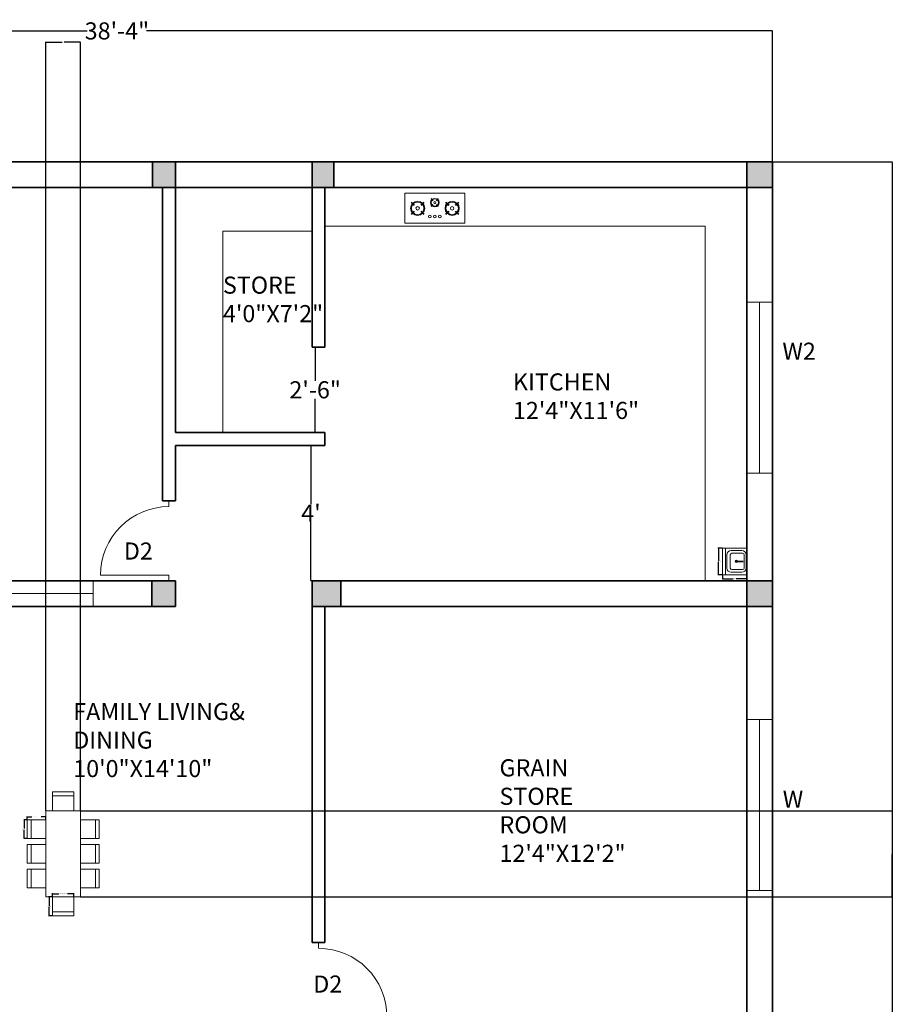
# Model space of a CAD drawing. Units: inches. Extents: x -36302355 to 648, y -221479757 to 75.
# Tile 37 of 37: x 341 to 648, y -271 to 75. Entities that reach past the tile are written whole.
import ezdxf

# ---------------------------------------------------------------- set-up
doc = ezdxf.new("R2010")
doc.units = ezdxf.units.IN
doc.header["$MEASUREMENT"] = 0
for name, color, linetype, lineweight in [('A-ANNO-DIMS', 2, 'Continuous', 18), ('A-ANNO-IDEN', 7, 'Continuous', 18), ('A-AREA-IDEN', 7, 'Continuous', 18), ('A-COLS', 7, 'Continuous', 35), ('A-COLS-PATT', 242, 'Continuous', 13), ('A-DOOR', 4, 'Continuous', 18), ('A-EQPM', 9, 'Continuous', 13), ('A-FLOR-CASE', 9, 'Continuous', 18), ('A-FLOR-FIXT', 9, 'Continuous', 18), ('A-FURN', 8, 'Continuous', 13), ('A-GLAZ', 142, 'Continuous', 18), ('A-WALL', 7, 'Continuous', 35)]:
    doc.layers.add(name, color=color, linetype=linetype, lineweight=lineweight)
doc.styles.get("Standard").update_dxf_attribs({"font": 'arial.ttf'})
doc.dimstyles.get("Standard").update_dxf_attribs({"dimtxt": 0.18, "dimasz": 0.18, "dimexe": 0.18, "dimexo": 0.0625, "dimgap": 0.09, "dimtad": 0, "dimtih": 1, "dimtoh": 1, "dimdec": 0, "dimzin": 0, "dimdsep": 46, "dimlunit": 3, "dimtxsty": 'Standard', "dimcen": 0.09, "dimadec": 0, "dimazin": 0, "dimtfac": 1, "dimtdec": 0, "dimtofl": 0, "dimtmove": 0, "dimatfit": 3, "dimfxl": 1, "dimtolj": 1, "dimtzin": 0, "dimarcsym": 0})

# ---------------------------------------------------------------- blocks, each defined once
blk = doc.blocks.new('*D2')
at = {"layer": 'A-ANNO-DIMS', "color": 0, "lineweight": -2, "transparency": 16777216}
for p, q in [((448.13, -74.52), (443.1, -74.52)), ((443.28, -74.7), (443.28, -95.18)), ((443.28, -121.84), (443.28, -101.36)), ((443.63, -122.02), (443.1, -122.02))]:
    blk.add_line(p, q, dxfattribs=at)
at = {"layer": 'A-ANNO-DIMS', "color": 0, "transparency": 16777216}
for points in [[(443.25, -74.7), (443.31, -74.7), (443.28, -74.52)], [(443.25, -121.84), (443.31, -121.84), (443.28, -122.02)]]:
    blk.add_solid(points, dxfattribs=at)
at = {"layer": 'Defpoints', "color": 0, "transparency": 16777216}
for p in [(448.2, -74.52), (443.28, -122.02), (443.7, -122.02)]:
    blk.add_point(p, dxfattribs=at)
at = {"layer": 'A-ANNO-DIMS', "color": 0, "transparency": 16777216, "insert": (443.28, -98.27), "char_height": 6, "attachment_point": 5}
blk.add_mtext("\\A1;4'", dxfattribs=at)
blk = doc.blocks.new('*D3')
at = {"layer": 'A-ANNO-DIMS', "color": 0, "lineweight": -2, "transparency": 16777216}
for p, q in [((445.88, -40.02), (444.57, -40.02)), ((444.75, -40.2), (444.75, -51.87)), ((444.75, -69.84), (444.75, -58.17)), ((445.88, -70.02), (444.57, -70.02))]:
    blk.add_line(p, q, dxfattribs=at)
at = {"layer": 'A-ANNO-DIMS', "color": 0, "transparency": 16777216}
for points in [[(444.72, -40.2), (444.78, -40.2), (444.75, -40.02)], [(444.72, -69.84), (444.78, -69.84), (444.75, -70.02)]]:
    blk.add_solid(points, dxfattribs=at)
at = {"layer": 'Defpoints', "color": 0, "transparency": 16777216}
for p in [(445.95, -40.02), (444.75, -70.02), (445.95, -70.02)]:
    blk.add_point(p, dxfattribs=at)
at = {"layer": 'A-ANNO-DIMS', "color": 0, "transparency": 16777216, "insert": (444.75, -55.02), "char_height": 6, "attachment_point": 5}
blk.add_mtext('\\A1;2\'-6"', dxfattribs=at)
blk = doc.blocks.new('*D4')
at = {"layer": 'A-ANNO-DIMS', "color": 0, "lineweight": -2, "transparency": 16777216}
for p, q in [((145.2, 25.04), (145.2, 71.11)), ((145.38, 70.93), (364.8, 70.93)), ((605.02, 70.93), (385.59, 70.93)), ((605.2, 25.04), (605.2, 71.11))]:
    blk.add_line(p, q, dxfattribs=at)
at = {"layer": 'A-ANNO-DIMS', "color": 0, "transparency": 16777216}
for points in [[(145.38, 70.96), (145.38, 70.9), (145.2, 70.93)], [(605.02, 70.96), (605.02, 70.9), (605.2, 70.93)]]:
    blk.add_solid(points, dxfattribs=at)
at = {"layer": 'Defpoints', "color": 0, "transparency": 16777216}
for p in [(605.2, 70.93), (145.2, 24.98), (605.2, 24.98)]:
    blk.add_point(p, dxfattribs=at)
at = {"layer": 'A-ANNO-DIMS', "color": 0, "transparency": 16777216, "insert": (375.2, 70.93), "char_height": 6, "attachment_point": 5}
blk.add_mtext('\\A1;38\'-4"', dxfattribs=at)
blk = doc.blocks.new('М14 600х655')
for p, q in [((-655, 600), (-655, 0)), ((-655, 600), (-655, 0)), ((-655, 0), (-655, 600)), ((0, 600), (-655, 600)), ((0, 525), (-655, 525)), ((-165, 494), (-490, 494)), ((0, 0), (0, 600)), ((-596, 388), (-596, 121)), ((-528, 370), (-528, 103)), ((-165, 408), (-490, 408)), ((-127, 103), (-127, 370)), ((-59, 121), (-59, 388)), ((-655, 0), (-655, 0)), ((-655, 0), (-655, 0)), ((-655, 0), (0, 0)), ((-655, 0), (0, 0)), ((-490, 65), (-165, 65)), ((-490, 15), (-165, 15)), ((-334, 87), (-334, 220)), ((-321, 87), (-321, 220))]:
    blk.add_line(p, q)
for radius in [27.6, 19.3]:
    blk.add_circle((-327, 259), radius)
for centre, radius, start, end in [((-490, 388), 106, 90, 180), ((-165, 388), 106, 0, 90), ((-490, 370), 38.2, 90, 180), ((-165, 370), 38.2, 0, 90), ((-490, 121), 106, 180, 270), ((-490, 103), 38.2, 180, 270), ((-165, 121), 106, 270, 0), ((-165, 103), 38.2, 270, 0)]:
    blk.add_arc(centre, radius, start, end)
blk = doc.blocks.new('WIN-60')
for p, q in [((60, 9), (0, 9)), ((0, 9), (0, 0)), ((60, 0), (60, 9)), ((0, 4.5), (60, 4.5)), ((0, 0), (60, 0))]:
    blk.add_line(p, q)
blk = doc.blocks.new('DOOR-SWING-24')
for p, q in [((0, 26), (0, 28)), ((0, 0), (0, 2)), ((0, 2), (24, 2))]:
    blk.add_line(p, q)
blk.add_arc((0, 2), 24, 0, 90)
blk = doc.blocks.new('CHAIR-DINING-SIDE')
for p, q in [((0, 6.6), (6.6, 6.6)), ((0, 0), (0, 6.6)), ((1.38, 6.6), (1.38, 0)), ((6.6, 0), (0, 0))]:
    blk.add_line(p, q)
blk = doc.blocks.new('CHAIR-DINING-END')
for p, q in [((0, 0), (0, 6.6)), ((7.57, 6.6), (7.57, 0)), ((0, 1.38), (7.57, 1.38)), ((7.57, 0), (0, 0))]:
    blk.add_line(p, q)
blk = doc.blocks.new('*D27')
at = {"layer": 'A-ANNO-DIMS', "color": 0, "lineweight": -2, "transparency": 16777216}
for p, q in [((343.68, -205.83), (343.68, -204.72)), ((343.86, -204.9), (345.38, -204.9)), ((350.11, -204.9), (348.59, -204.9)), ((350.29, -205.83), (350.29, -204.72))]:
    blk.add_line(p, q, dxfattribs=at)
at = {"layer": 'A-ANNO-DIMS', "color": 0, "transparency": 16777216}
for points in [[(343.86, -204.87), (343.86, -204.93), (343.68, -204.9)], [(350.11, -204.87), (350.11, -204.93), (350.29, -204.9)]]:
    blk.add_solid(points, dxfattribs=at)
at = {"layer": 'Defpoints', "color": 0, "transparency": 16777216}
for p in [(343.68, -205.89), (350.29, -204.9), (350.29, -205.89)]:
    blk.add_point(p, dxfattribs=at)
at = {"layer": 'A-ANNO-DIMS', "color": 0, "transparency": 16777216, "insert": (346.99, -204.9), "char_height": 0.18, "attachment_point": 5}
blk.add_mtext('\\A1;SIDE CHAIR 0\'-6 1/2" TYP.', dxfattribs=at)
blk = doc.blocks.new('*D28')
at = {"layer": 'A-ANNO-DIMS', "color": 0, "lineweight": -2, "transparency": 16777216}
for p, q in [((343.62, -205.89), (342.51, -205.89)), ((342.69, -206.07), (342.69, -209.01)), ((342.69, -212.31), (342.69, -209.38)), ((343.62, -212.49), (342.51, -212.49))]:
    blk.add_line(p, q, dxfattribs=at)
at = {"layer": 'A-ANNO-DIMS', "color": 0, "transparency": 16777216}
for points in [[(342.66, -206.07), (342.72, -206.07), (342.69, -205.89)], [(342.66, -212.31), (342.72, -212.31), (342.69, -212.49)]]:
    blk.add_solid(points, dxfattribs=at)
at = {"layer": 'Defpoints', "color": 0, "transparency": 16777216}
for p in [(342.69, -205.89), (343.68, -205.89), (343.68, -212.49)]:
    blk.add_point(p, dxfattribs=at)
at = {"layer": 'A-ANNO-DIMS', "color": 0, "transparency": 16777216, "insert": (342.69, -209.19), "char_height": 0.18, "attachment_point": 5}
blk.add_mtext('\\A1;0\'-6 1/2" TYP.', dxfattribs=at)
blk = doc.blocks.new('*D33')
at = {"layer": 'A-ANNO-DIMS', "color": 0, "lineweight": -2, "transparency": 16777216}
for p, q in [((587.6, -110.59), (586.08, -110.59)), ((586.26, -110.77), (586.26, -115.07)), ((586.26, -119.73), (586.26, -115.44)), ((587.6, -119.91), (586.08, -119.91))]:
    blk.add_line(p, q, dxfattribs=at)
at = {"layer": 'A-ANNO-DIMS', "color": 0, "transparency": 16777216}
for points in [[(586.23, -110.77), (586.29, -110.77), (586.26, -110.59)], [(586.23, -119.73), (586.29, -119.73), (586.26, -119.91)]]:
    blk.add_solid(points, dxfattribs=at)
at = {"layer": 'Defpoints', "color": 0, "transparency": 16777216}
for p in [(586.26, -110.59), (587.66, -110.59), (587.66, -119.91)]:
    blk.add_point(p, dxfattribs=at)
at = {"layer": 'A-ANNO-DIMS', "color": 0, "transparency": 16777216, "insert": (586.26, -115.25), "char_height": 0.18, "attachment_point": 5}
blk.add_mtext('\\A1;BASIN 0\'-9 1/2"', dxfattribs=at)
blk = doc.blocks.new('*D34')
at = {"layer": 'A-ANNO-DIMS', "color": 0, "lineweight": -2, "transparency": 16777216}
for p, q in [((587.66, -119.97), (587.66, -121.49)), ((596.2, -119.97), (596.2, -121.49)), ((587.84, -121.31), (591.39, -121.31)), ((596.02, -121.31), (592.47, -121.31))]:
    blk.add_line(p, q, dxfattribs=at)
at = {"layer": 'A-ANNO-DIMS', "color": 0, "transparency": 16777216}
for points in [[(587.84, -121.28), (587.84, -121.34), (587.66, -121.31)], [(596.02, -121.28), (596.02, -121.34), (596.2, -121.31)]]:
    blk.add_solid(points, dxfattribs=at)
at = {"layer": 'Defpoints', "color": 0, "transparency": 16777216}
for p in [(587.66, -119.91), (596.2, -119.91), (587.66, -121.31)]:
    blk.add_point(p, dxfattribs=at)
at = {"layer": 'A-ANNO-DIMS', "color": 0, "transparency": 16777216, "insert": (591.93, -121.31), "char_height": 0.18, "attachment_point": 5}
blk.add_mtext('\\A1;0\'-8 1/2"', dxfattribs=at)
blk = doc.blocks.new('*D53')
at = {"layer": 'A-ANNO-DIMS', "color": 0, "lineweight": -2, "transparency": 16777216}
for p, q in [((352.56, -232.93), (352.56, -231.68)), ((352.74, -231.86), (354.77, -231.86)), ((359.94, -231.86), (357.91, -231.86)), ((360.12, -232.93), (360.12, -231.68))]:
    blk.add_line(p, q, dxfattribs=at)
at = {"layer": 'A-ANNO-DIMS', "color": 0, "transparency": 16777216}
for points in [[(352.74, -231.83), (352.74, -231.89), (352.56, -231.86)], [(359.94, -231.83), (359.94, -231.89), (360.12, -231.86)]]:
    blk.add_solid(points, dxfattribs=at)
at = {"layer": 'Defpoints', "color": 0, "transparency": 16777216}
for p in [(352.56, -232.99), (360.12, -231.86), (360.12, -232.99)]:
    blk.add_point(p, dxfattribs=at)
at = {"layer": 'A-ANNO-DIMS', "color": 0, "transparency": 16777216, "insert": (356.34, -231.86), "char_height": 0.18, "attachment_point": 5}
blk.add_mtext('\\A1;END CHAIR 0\'-7 1/2" TYP.', dxfattribs=at)
blk = doc.blocks.new('*D54')
at = {"layer": 'A-ANNO-DIMS', "color": 0, "lineweight": -2, "transparency": 16777216}
for p, q in [((352.49, -232.99), (351.24, -232.99)), ((351.42, -233.17), (351.42, -236.11)), ((351.42, -239.41), (351.42, -236.48)), ((352.49, -239.59), (351.24, -239.59))]:
    blk.add_line(p, q, dxfattribs=at)
at = {"layer": 'A-ANNO-DIMS', "color": 0, "transparency": 16777216}
for points in [[(351.39, -233.17), (351.45, -233.17), (351.42, -232.99)], [(351.39, -239.41), (351.45, -239.41), (351.42, -239.59)]]:
    blk.add_solid(points, dxfattribs=at)
at = {"layer": 'Defpoints', "color": 0, "transparency": 16777216}
for p in [(351.42, -232.99), (352.56, -232.99), (352.56, -239.59)]:
    blk.add_point(p, dxfattribs=at)
at = {"layer": 'A-ANNO-DIMS', "color": 0, "transparency": 16777216, "insert": (351.42, -236.29), "char_height": 0.18, "attachment_point": 5}
blk.add_mtext('\\A1;0\'-6 1/2" TYP.', dxfattribs=at)
blk = doc.blocks.new('*D57')
at = {"layer": 'A-ANNO-DIMS', "color": 0, "lineweight": -2, "transparency": 16777216}
for p, q in [((605.26, 24.98), (647.33, 24.98)), ((647.15, 24.8), (647.15, -348.34)), ((647.15, -721.84), (647.15, -348.7)), ((605.26, -722.02), (647.33, -722.02))]:
    blk.add_line(p, q, dxfattribs=at)
at = {"layer": 'A-ANNO-DIMS', "color": 0, "transparency": 16777216}
for points in [[(647.12, 24.8), (647.18, 24.8), (647.15, 24.98)], [(647.12, -721.84), (647.18, -721.84), (647.15, -722.02)]]:
    blk.add_solid(points, dxfattribs=at)
at = {"layer": 'Defpoints', "color": 0, "transparency": 16777216}
for p in [(605.2, 24.98), (605.2, -722.02), (647.15, -722.02)]:
    blk.add_point(p, dxfattribs=at)
at = {"layer": 'A-ANNO-DIMS', "color": 0, "transparency": 16777216, "insert": (647.15, -348.52), "char_height": 0.18, "attachment_point": 5}
blk.add_mtext('\\A1;62\'-3"', dxfattribs=at)
blk = doc.blocks.new('*D58')
at = {"layer": 'A-ANNO-DIMS', "color": 0, "lineweight": -2, "transparency": 16777216}
for p, q in [((350.29, -202.66), (350.29, 67.11)), ((350.47, 66.93), (356.02, 66.93)), ((362.21, 66.93), (356.66, 66.93)), ((362.39, -202.66), (362.39, 67.11))]:
    blk.add_line(p, q, dxfattribs=at)
at = {"layer": 'A-ANNO-DIMS', "color": 0, "transparency": 16777216}
for points in [[(350.47, 66.96), (350.47, 66.9), (350.29, 66.93)], [(362.21, 66.96), (362.21, 66.9), (362.39, 66.93)]]:
    blk.add_solid(points, dxfattribs=at)
at = {"layer": 'Defpoints', "color": 0, "transparency": 16777216}
for p in [(362.39, 66.93), (350.29, -202.73), (362.39, -202.73)]:
    blk.add_point(p, dxfattribs=at)
at = {"layer": 'A-ANNO-DIMS', "color": 0, "transparency": 16777216, "insert": (356.34, 66.93), "char_height": 0.18, "attachment_point": 5}
blk.add_mtext('\\A1;1\'-0"', dxfattribs=at)
blk = doc.blocks.new('*D59')
at = {"layer": 'A-ANNO-DIMS', "color": 0, "lineweight": -2, "transparency": 16777216}
for p, q in [((362.45, -202.73), (647.33, -202.73)), ((647.15, -202.91), (647.15, -217.68)), ((647.15, -232.81), (647.15, -218.04)), ((362.45, -232.99), (647.33, -232.99))]:
    blk.add_line(p, q, dxfattribs=at)
at = {"layer": 'A-ANNO-DIMS', "color": 0, "transparency": 16777216}
for points in [[(647.12, -202.91), (647.18, -202.91), (647.15, -202.73)], [(647.12, -232.81), (647.18, -232.81), (647.15, -232.99)]]:
    blk.add_solid(points, dxfattribs=at)
at = {"layer": 'Defpoints', "color": 0, "transparency": 16777216}
for p in [(362.39, -202.73), (362.39, -232.99), (647.15, -232.99)]:
    blk.add_point(p, dxfattribs=at)
at = {"layer": 'A-ANNO-DIMS', "color": 0, "transparency": 16777216, "insert": (647.15, -217.86), "char_height": 0.18, "attachment_point": 5}
blk.add_mtext('\\A1;2\'-6 1/2"', dxfattribs=at)

msp = doc.modelspace()

# ---------------------------------------------------------------- hatches: boundary and pattern name
at = {"layer": 'A-COLS-PATT'}
h = msp.add_hatch(color=256, dxfattribs=at)
h.dxf.hatch_style = 1
h.paths.add_polyline_path([(145.2, 24.98), (145.2, 15.98), (154.2, 15.98), (154.2, 24.98)])
h.paths.add_polyline_path([(247.2, 15.98), (247.2, 24.98), (238.2, 24.98), (238.2, 15.98)])
h.paths.add_polyline_path([(387.64, 15.98), (395.7, 15.98), (395.7, 24.98), (387.64, 24.98)])
h.paths.add_polyline_path([(451.26, 24.98), (443.7, 24.98), (443.7, 15.98), (451.26, 15.98)])
h.paths.add_polyline_path([(596.2, 15.98), (605.2, 15.98), (605.2, 24.98), (596.2, 24.98)])
h.paths.add_polyline_path([(238.2, -122.02), (238.2, -131.02), (247.2, -131.02), (247.2, -122.02)])
h.paths.add_polyline_path([(395.7, -122.02), (387.46, -122.02), (387.46, -131.02), (395.7, -131.02)])
h.paths.add_polyline_path([(448.2, -131.02), (453.73, -131.02), (453.73, -122.02), (443.7, -122.02), (443.7, -131.02)])
h.paths.add_polyline_path([(596.2, -131.02), (605.2, -131.02), (605.2, -122.02), (596.2, -122.02)])
h.paths.add_polyline_path([(145.2, -176.97), (154.2, -176.97), (154.2, -167.02), (145.2, -167.02)])
h.paths.add_polyline_path([(314.2, -176.97), (323.2, -176.97), (323.2, -167.02), (314.2, -167.02)])
h.paths.add_polyline_path([(154.2, -314.02), (154.2, -309.52), (145.2, -309.52), (145.2, -314.02)])
h.paths.add_polyline_path([(314.2, -309.52), (314.2, -318.52), (323.2, -318.52), (323.2, -309.52)])
h.paths.add_polyline_path([(448.2, -277.02), (443.7, -277.02), (443.7, -286.02), (448.2, -286.02)])
h.paths.add_polyline_path([(283.2, -370.02), (274.2, -370.02), (274.2, -379.02), (283.2, -379.02), (283.2, -374.52)])
h.paths.add_polyline_path([(154.2, -370.02), (145.2, -370.02), (145.2, -379.02), (154.2, -379.02)])
h.paths.add_polyline_path([(443.2, -374.52), (443.2, -379.02), (452.2, -379.02), (452.2, -374.52)])
h.paths.add_polyline_path([(145.2, -580.02), (154.2, -580.02), (154.2, -571.02), (145.2, -571.02)])
h.paths.add_polyline_path([(274.2, -571.02), (274.2, -580.02), (283.2, -580.02), (283.2, -571.02)])
h.paths.add_polyline_path([(443.2, -580.02), (452.2, -580.02), (452.2, -571.02), (443.2, -571.02)])

# ---------------------------------------------------------------- linework, layer by layer
at = {"layer": 'A-COLS'}
for p, q in [((387.64, 24.98), (387.64, 15.98)), ((451.26, 24.98), (451.26, 15.98)), ((387.46, -122.02), (387.46, -131.02)), ((395.7, -122.02), (395.7, -131.02)), ((443.7, -122.02), (448.2, -122.02)), ((443.7, -131.02), (443.7, -122.02)), ((453.73, -122.02), (453.73, -131.02)), ((443.7, -131.02), (448.2, -131.02))]:
    msp.add_line(p, q, dxfattribs=at)
at = {"layer": 'A-EQPM'}
for p, q in [((497.31, 14), (476.22, 14)), ((476.22, 14), (476.22, 3.45)), ((497.31, 3.45), (497.31, 14)), ((479.47, 9.62), (478.38, 10.72)), ((479.62, 9.77), (478.52, 10.86)), ((481.8, 9.78), (482.89, 10.88)), ((481.94, 9.63), (483.03, 10.74)), ((486.06, 11.33), (485.4, 11.99)), ((486.15, 11.42), (485.49, 12.08)), ((487.28, 11.42), (487.94, 12.08)), ((487.37, 11.33), (488.03, 11.99)), ((491.59, 9.63), (490.5, 10.74)), ((491.74, 9.78), (490.65, 10.88)), ((493.92, 9.77), (495.01, 10.86)), ((494.06, 9.62), (495.16, 10.72)), ((479.47, 7.73), (478.38, 6.63)), ((479.62, 7.58), (478.52, 6.48)), ((481.8, 7.57), (482.89, 6.47)), ((481.94, 7.72), (483.03, 6.61)), ((486.06, 10.03), (485.39, 9.37)), ((486.14, 9.94), (485.48, 9.28)), ((487.29, 9.94), (487.95, 9.28)), ((487.38, 10.03), (488.04, 9.37)), ((491.59, 7.72), (490.5, 6.61)), ((491.74, 7.57), (490.65, 6.47)), ((493.92, 7.58), (495.01, 6.48)), ((494.06, 7.73), (495.16, 6.63)), ((476.22, 3.45), (497.31, 3.45))]:
    msp.add_line(p, q, dxfattribs=at)
for centre, radius in [((480.71, 8.67), 2.48), ((480.71, 8.67), 2.18), ((486.72, 10.68), 1.49), ((486.72, 10.68), 1.31), ((486.72, 10.68), 0.383), ((492.82, 8.67), 2.48), ((492.82, 8.67), 2.18), ((480.71, 8.67), 0.639), ((492.82, 8.67), 0.639), ((485.01, 5.8), 0.469), ((486.77, 5.8), 0.469), ((488.52, 5.8), 0.469)]:
    msp.add_circle(centre, radius, dxfattribs=at)
at = {"layer": 'A-FLOR-CASE'}
for p, q in [((443.7, 0.64), (412.39, 0.64)), ((412.39, 0.64), (412.39, -70.02)), ((448.2, 2.38), (581.58, 2.38)), ((581.58, 2.38), (581.58, -122.02))]:
    msp.add_line(p, q, dxfattribs=at)
at = {"layer": 'A-FURN'}
for p, q in [((350.29, -232.99), (350.29, -202.73)), ((350.29, -202.73), (362.39, -202.73)), ((362.39, -202.73), (362.39, -232.99)), ((362.39, -232.99), (350.29, -232.99))]:
    msp.add_line(p, q, dxfattribs=at)
at = {"layer": 'A-WALL'}
for p, q in [((145.2, 24.98), (605.2, 24.98)), ((395.7, 24.98), (395.7, -70.02)), ((443.7, 24.98), (443.7, -40.02)), ((596.2, 24.98), (596.2, -426.52)), ((605.2, 24.98), (605.2, -722.02)), ((145.2, 15.98), (605.2, 15.98)), ((391.2, 15.98), (391.2, -94.02)), ((448.2, 15.98), (448.2, -40.02)), ((443.7, -40.02), (448.2, -40.02)), ((395.7, -70.02), (448.2, -70.02)), ((448.2, -70.02), (448.2, -74.52)), ((395.7, -74.52), (448.2, -74.52)), ((395.7, -74.52), (395.7, -94.02)), ((393.45, -94.02), (391.2, -94.02)), ((393.45, -94.02), (395.7, -94.02)), ((238.2, -122.02), (395.7, -122.02)), ((443.7, -122.02), (605.2, -122.02)), ((238.2, -131.02), (395.7, -131.02)), ((443.7, -131.02), (443.7, -249.02)), ((443.7, -131.02), (605.2, -131.02)), ((448.2, -131.02), (448.2, -249.02)), ((445.95, -249.02), (443.7, -249.02)), ((445.95, -249.02), (448.2, -249.02))]:
    msp.add_line(p, q, dxfattribs=at)

# ---------------------------------------------------------------- block references
at = {"layer": 'A-DOOR', "extrusion": (0, 0, -1), "zscale": -1}
msp.add_blockref('DOOR-SWING-24', (-393.45, -122.02), dxfattribs=at)
at = {"layer": 'A-DOOR'}
msp.add_blockref('DOOR-SWING-24', (445.95, -277.02), dxfattribs=at)
at = {"layer": 'A-FLOR-FIXT', "xscale": 0.0142252425150931, "yscale": 0.0142252425150931, "zscale": 0.0142252425150931, "rotation": 90}
msp.add_blockref('М14 600х655', (596.2, -110.59), dxfattribs=at)
at = {"layer": 'A-FURN', "extrusion": (0, 0, -1), "zscale": -1, "rotation": 180}
msp.add_blockref('CHAIR-DINING-END', (-352.56, -196.12), dxfattribs=at)
at = {"layer": 'A-FURN'}
for name, p in [('CHAIR-DINING-SIDE', (343.68, -212.49)), ('CHAIR-DINING-SIDE', (343.68, -221.16)), ('CHAIR-DINING-SIDE', (343.68, -229.83)), ('CHAIR-DINING-END', (352.56, -239.59))]:
    msp.add_blockref(name, p, dxfattribs=at)
at = {"layer": 'A-FURN', "extrusion": (0, 0, -1), "zscale": -1}
for p in [(-369, -212.49), (-369, -221.16), (-369, -229.83)]:
    msp.add_blockref('CHAIR-DINING-SIDE', p, dxfattribs=at)
at = {"layer": 'A-GLAZ', "extrusion": (0, 0, -1), "zscale": -1, "rotation": 90}
for p in [(-596.2, -84.24), (-596.2, -230.77)]:
    msp.add_blockref('WIN-60', p, dxfattribs=at)
at = {"layer": 'A-GLAZ'}
msp.add_blockref('WIN-60', (306.86, -131.02), dxfattribs=at)

# ---------------------------------------------------------------- texts
at = {"layer": 'A-ANNO-IDEN', "insert": (608.7, -38.48), "char_height": 6, "attachment_point": 1}
msp.add_mtext_dynamic_manual_height_columns('W2', width=5.8138, gutter_width=1, heights=[0], dxfattribs=at)
at = {"layer": 'A-ANNO-IDEN', "char_height": 6, "attachment_point": 1}
for s, insert in [('D2', (377.63, -108.6)), ('W', (608.81, -195.68)), ('D2', (444.08, -260.56))]:
    msp.add_mtext(s, dxfattribs=dict(at, insert=insert))
at = {"layer": 'A-AREA-IDEN', "insert": (412.39, -15.28), "char_height": 6, "attachment_point": 1}
msp.add_mtext_dynamic_manual_height_columns('STORE\\P4\'0"X7\'2"', width=2.6178, gutter_width=1, heights=[0], dxfattribs=at)
at = {"layer": 'A-AREA-IDEN', "char_height": 6, "attachment_point": 1}
for s, insert in [('KITCHEN\\P12\'4"X11\'6"', (514.15, -49.26)), ('FAMILY LIVING&\\PDINING\\P10\'0"X14\'10"', (359.87, -164.94)), ('GRAIN\\PSTORE\\PROOM\\P12\'4"X12\'2"', (509.42, -184.67))]:
    msp.add_mtext(s, dxfattribs=dict(at, insert=insert))

# ---------------------------------------------------------------- dimensions: what is measured, and where the dimension line sits
at = {"layer": 'A-ANNO-DIMS'}
for base, p1, p2, override, picture, middle in [((605.2, 70.93), (145.2, 24.98), (605.2, 24.98), {"dimtxt": 6, "dimclrd": 0, "dimclre": 0, "dimclrt": 0}, '*D4', (375.2, 70.93)), ((362.39, 66.93), (350.29, -202.73), (362.39, -202.73), {"dimdec": 1, "dimlfac": 1, "dimrnd": 0, "dimzin": 1, "dimdsep": 46, "dimlunit": 4, "dimfrac": 2}, '*D58', (356.34, 66.93))]:
    dim = msp.add_linear_dim(base=base, p1=p1, p2=p2, dimstyle='Standard', override=override, dxfattribs=at)
    dim.commit()
    dim.dimension.update_dxf_attribs({"geometry": picture, "text_midpoint": middle})
for base, p1, p2, angle, override, picture, middle in [((647.15, -722.02), (605.2, 24.98), (605.2, -722.02), 90, {"dimdec": 1, "dimlfac": 1, "dimrnd": 0, "dimzin": 1, "dimdsep": 46, "dimlunit": 4, "dimfrac": 2}, '*D57', (647.15, -348.52)), ((444.75, -70.02), (445.95, -40.02), (445.95, -70.02), 90, {"dimtxt": 6, "dimclrd": 0, "dimclre": 0, "dimclrt": 0}, '*D3', (444.75, -55.02)), ((443.27639282, -122.01917599), (448.19674998, -74.51917599), (443.69674998, -122.01917599), 90, {"dimtxt": 6, "dimclrd": 0, "dimclre": 0, "dimclrt": 0}, '*D2', (443.27639282, -98.26917599)), ((587.66, -121.31), (596.2, -119.91), (587.66, -119.91), 180, {"dimdec": 1, "dimlfac": 1, "dimrnd": 0, "dimzin": 1, "dimdsep": 46, "dimlunit": 4, "dimfrac": 2}, '*D34', (591.93, -121.31)), ((647.15, -232.99), (362.39, -202.73), (362.39, -232.99), 90, {"dimdec": 1, "dimlfac": 1, "dimrnd": 0, "dimzin": 1, "dimdsep": 46, "dimlunit": 4, "dimfrac": 2}, '*D59', (647.15, -217.86))]:
    dim = msp.add_linear_dim(base=base, p1=p1, p2=p2, angle=angle, dimstyle='Standard', override=override, dxfattribs=at)
    dim.commit()
    dim.dimension.update_dxf_attribs({"geometry": picture, "text_midpoint": middle})
for base, p1, p2, text, picture, middle in [((586.26, -110.59), (587.66, -119.91), (587.66, -110.59), 'BASIN <>', '*D33', (586.26, -115.25)), ((342.69, -205.89), (343.68, -212.49), (343.68, -205.89), '<> TYP.', '*D28', (342.69, -209.19)), ((351.42, -232.99), (352.56, -239.59), (352.56, -232.99), '<> TYP.', '*D54', (351.42, -236.29))]:
    dim = msp.add_linear_dim(base=base, p1=p1, p2=p2, angle=90, text=text, dimstyle='Standard', override={"dimdec": 1, "dimlfac": 1, "dimrnd": 0, "dimzin": 1, "dimdsep": 46, "dimlunit": 4, "dimfrac": 2}, dxfattribs=at)
    dim.commit()
    dim.dimension.update_dxf_attribs({"geometry": picture, "text_midpoint": middle})
for base, p1, p2, text, picture, middle in [((350.29, -204.9), (343.68, -205.89), (350.29, -205.89), 'SIDE CHAIR <> TYP.', '*D27', (346.99, -204.9)), ((360.12, -231.86), (352.56, -232.99), (360.12, -232.99), 'END CHAIR <> TYP.', '*D53', (356.34, -231.86))]:
    dim = msp.add_linear_dim(base=base, p1=p1, p2=p2, text=text, dimstyle='Standard', override={"dimdec": 1, "dimlfac": 1, "dimrnd": 0, "dimzin": 1, "dimdsep": 46, "dimlunit": 4, "dimfrac": 2}, dxfattribs=at)
    dim.commit()
    dim.dimension.update_dxf_attribs({"geometry": picture, "text_midpoint": middle})

doc.saveas('drawing.dxf')
